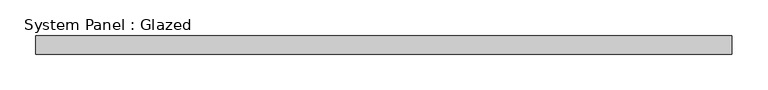
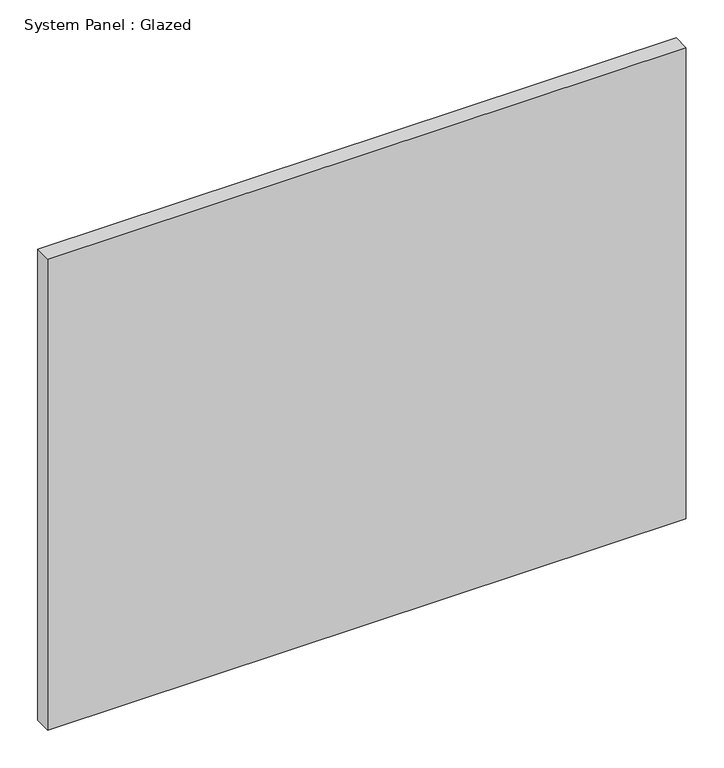
"""IFC4 building model written with IfcOpenShell, lengths in millimetres: plate geometry, System Panel : Glazed."""

from ifc_helpers import new_model, si_unit, origin, origin_with_axes, place, context, project, spatial, polyline, outline, extrude, source, transform, mapped, element, save


def system_panel_glazed_e22b6634(model_context):
    return source(origin(), model_context, "Body", "SweptSolid", [
        extrude(outline(polyline([(485.775, 19.05), (-485.775, 19.05), (-485.775, 44.45), (485.775, 44.45), (485.775, 19.05)])), origin_with_axes(), (0.0, 0.0, 1.0), 757.5270145),
    ])


if __name__ == "__main__":
    model = new_model("IFC4")
    model_context = context("Model", 3, world=origin())
    ifc_project = project(units=[si_unit("LENGTHUNIT", "METRE", prefix="MILLI")], contexts=[model_context])
    site = spatial("IfcSite", under=ifc_project)
    building = spatial("IfcBuilding", under=site)
    placement = place(None, origin())
    system_panel_glazed_shape = system_panel_glazed_e22b6634(model_context)
    element("IfcPlate", 1, ObjectType="System Panel : Glazed", at=placement, inside=building, context=model_context, shape_type="MappedRepresentation", body=[
        mapped(system_panel_glazed_shape, transform((0.0, 0.0, 0.0), x_axis=(1.0, 0.0, 0.0), y_axis=(0.0, 1.0, 0.0), z_axis=(0.0, 0.0, 1.0))),
    ])
    save(model, "model.ifc")

# Revit data of these elements
# Type "System Panel : Glazed"
#   Construction Type Id = "GSP4R"
#   Analytic Construction = "1/8 in Pilkington single glazing"
#   Visual Light Transmittance = 0.9
#   Solar Heat Gain Coefficient = 0.86
#   Heat Transfer Coefficient (U) = 1.18115 BTU/(h·ft²·°F)
#   Define Thermal Properties by = 1
# Element 1 (IfcPlate, "System Panel : Glazed")
#   Materials on its faces: "Glass"
# Materials
#   "Glass": class "Glass", colour RGB 0 128 192, transparency 0.75, Description = "Soda Lime Glass", Cost = 0
